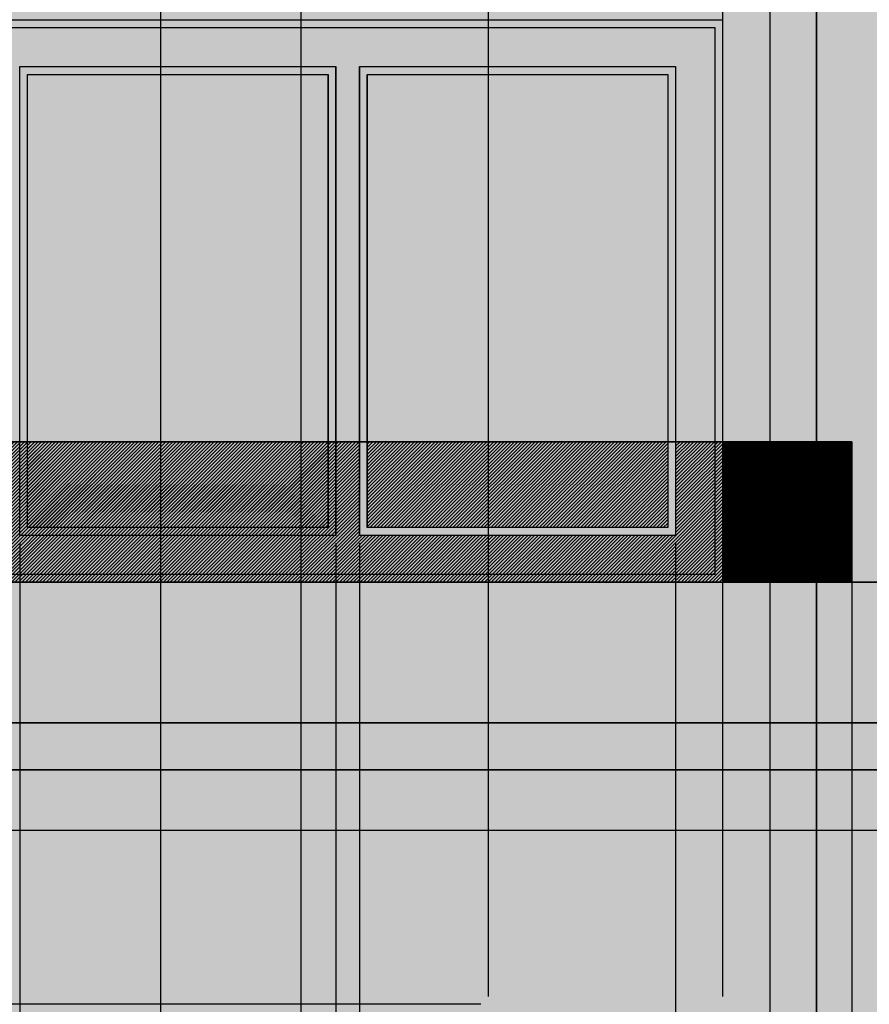
# Model space of a CAD drawing. Units: inches. Extents: x 860 to 1491, y 583 to 1370.
# Tile 5 of 8: x 998 to 1216, y 839 to 1091. Entities that reach past the tile are written whole.
import ezdxf

# ---------------------------------------------------------------- set-up
doc = ezdxf.new("R2010")
doc.units = ezdxf.units.IN
doc.header["$MEASUREMENT"] = 0
doc.layers.get('0').update_dxf_attribs({"color": 250})
for name, color, linetype, lineweight in [('A-ANNO-DIMS', 2, 'Continuous', 18), ('A-ELEV', 7, 'Continuous', 35), ('A-ELEV-PATT', 9, 'Continuous', 13), ('A-GLAZ', 4, 'Continuous', 25), ('A-GLAZ-PATT', 150, 'Continuous', 13), ('A-RAIL-PATT', 150, 'Continuous', 13)]:
    doc.layers.add(name, color=color, linetype=linetype, lineweight=lineweight)
doc.styles.get("Standard").update_dxf_attribs({"font": 'arial.ttf'})
doc.dimstyles.get("Standard").update_dxf_attribs({"dimtxt": 6, "dimasz": 0.18, "dimexe": 3, "dimexo": 2, "dimgap": 2, "dimtad": 0, "dimtih": 1, "dimtoh": 1, "dimdec": 0, "dimzin": 0, "dimdsep": 46, "dimlunit": 3, "dimtxsty": 'Standard', "dimblk2": 'CLOSEDBLANK', "dimsah": 1, "dimcen": 2, "dimadec": 0, "dimazin": 0, "dimtfac": 1, "dimtdec": 0, "dimtofl": 0, "dimtmove": 0, "dimatfit": 3, "dimfxl": 1, "dimtolj": 1, "dimtzin": 0, "dimarcsym": 0})

# ---------------------------------------------------------------- blocks, each defined once
blk = doc.blocks.new('_ClosedBlank')
at = {"color": 0, "linetype": 'ByBlock', "lineweight": -2}
for p, q in [((-1, 0.17), (0, 0)), ((-1, 0.17), (-1, -0.17)), ((0, 0), (-1, -0.17))]:
    blk.add_line(p, q, dxfattribs=at)
blk = doc.blocks.new('*D2')
at = {"layer": 'A-ANNO-DIMS', "color": 0, "lineweight": -2, "transparency": 16777216}
for p, q in [((1442.44, 1328.76), (1442.44, 584.11)), ((908.34, 740.76), (908.34, 584.11)), ((908.52, 587.11), (1163.85, 587.11)), ((1442.26, 587.11), (1186.93, 587.11))]:
    blk.add_line(p, q, dxfattribs=at)
at = {"layer": 'A-ANNO-DIMS', "color": 0, "transparency": 16777216}
blk.add_solid([(908.52, 587.14), (908.52, 587.08), (908.34, 587.11)], dxfattribs=at)
at = {"layer": 'Defpoints', "color": 0, "transparency": 16777216}
for p in [(1442.44, 1330.76), (908.34, 742.76), (1442.44, 587.11)]:
    blk.add_point(p, dxfattribs=at)
at = {"layer": 'A-ANNO-DIMS', "color": 0, "lineweight": -2, "transparency": 16777216, "xscale": 0.18, "yscale": 0.18, "zscale": 0.18}
blk.add_blockref('_ClosedBlank', (1442.44, 587.11), dxfattribs=at)
at = {"layer": 'A-ANNO-DIMS', "color": 0, "transparency": 16777216, "insert": (1175.39, 587.11), "char_height": 6, "attachment_point": 5}
blk.add_mtext('\\A1;534.1', dxfattribs=at)
blk = doc.blocks.new('*D21')
at = {"layer": 'A-ANNO-DIMS', "color": 0, "lineweight": -2, "transparency": 16777216}
for p, q in [((962.34, 732.76), (962.34, 1369.41)), ((1034.46, 828.76), (1034.46, 1369.41)), ((962.52, 1366.41), (986.33, 1366.41)), ((1034.28, 1366.41), (1010.47, 1366.41))]:
    blk.add_line(p, q, dxfattribs=at)
at = {"layer": 'A-ANNO-DIMS', "color": 0, "transparency": 16777216}
blk.add_solid([(962.52, 1366.44), (962.52, 1366.38), (962.34, 1366.41)], dxfattribs=at)
at = {"layer": 'Defpoints', "color": 0, "transparency": 16777216}
for p in [(1034.46, 1366.41), (1034.46, 826.76), (962.34, 730.76)]:
    blk.add_point(p, dxfattribs=at)
at = {"layer": 'A-ANNO-DIMS', "color": 0, "lineweight": -2, "transparency": 16777216, "xscale": 0.18, "yscale": 0.18, "zscale": 0.18}
blk.add_blockref('_ClosedBlank', (1034.46, 1366.41), dxfattribs=at)
at = {"layer": 'A-ANNO-DIMS', "color": 0, "transparency": 16777216, "insert": (998.4, 1366.41), "char_height": 6, "attachment_point": 5}
blk.add_mtext('\\A1;72.12', dxfattribs=at)
blk = doc.blocks.new('*D22')
at = {"layer": 'A-ANNO-DIMS', "color": 0, "lineweight": -2, "transparency": 16777216}
for p, q in [((1034.46, 828.76), (1034.46, 1369.41)), ((1070.46, 828.76), (1070.46, 1369.41)), ((1034.64, 1366.41), (1046.17, 1366.41)), ((1070.28, 1366.41), (1058.75, 1366.41))]:
    blk.add_line(p, q, dxfattribs=at)
at = {"layer": 'A-ANNO-DIMS', "color": 0, "transparency": 16777216}
blk.add_solid([(1034.64, 1366.44), (1034.64, 1366.38), (1034.46, 1366.41)], dxfattribs=at)
at = {"layer": 'Defpoints', "color": 0, "transparency": 16777216}
for p in [(1070.46, 1366.41), (1034.46, 826.76), (1070.46, 826.76)]:
    blk.add_point(p, dxfattribs=at)
at = {"layer": 'A-ANNO-DIMS', "color": 0, "lineweight": -2, "transparency": 16777216, "xscale": 0.18, "yscale": 0.18, "zscale": 0.18}
blk.add_blockref('_ClosedBlank', (1070.46, 1366.41), dxfattribs=at)
at = {"layer": 'A-ANNO-DIMS', "color": 0, "transparency": 16777216, "insert": (1052.46, 1366.41), "char_height": 6, "attachment_point": 5}
blk.add_mtext('\\A1;36', dxfattribs=at)
blk = doc.blocks.new('*D23')
at = {"layer": 'A-ANNO-DIMS', "color": 0, "lineweight": -2, "transparency": 16777216}
for p, q in [((1070.46, 828.76), (1070.46, 1369.41)), ((1118.44, 840.76), (1118.44, 1369.41)), ((1070.64, 1366.41), (1082.2, 1366.41)), ((1118.26, 1366.41), (1106.7, 1366.41))]:
    blk.add_line(p, q, dxfattribs=at)
at = {"layer": 'A-ANNO-DIMS', "color": 0, "transparency": 16777216}
blk.add_solid([(1070.64, 1366.44), (1070.64, 1366.38), (1070.46, 1366.41)], dxfattribs=at)
at = {"layer": 'Defpoints', "color": 0, "transparency": 16777216}
for p in [(1118.44, 1366.41), (1118.44, 838.76), (1070.46, 826.76)]:
    blk.add_point(p, dxfattribs=at)
at = {"layer": 'A-ANNO-DIMS', "color": 0, "lineweight": -2, "transparency": 16777216, "xscale": 0.18, "yscale": 0.18, "zscale": 0.18}
blk.add_blockref('_ClosedBlank', (1118.44, 1366.41), dxfattribs=at)
at = {"layer": 'A-ANNO-DIMS', "color": 0, "transparency": 16777216, "insert": (1094.45, 1366.41), "char_height": 6, "attachment_point": 5}
blk.add_mtext('\\A1;47.98', dxfattribs=at)
blk = doc.blocks.new('*D24')
at = {"layer": 'A-ANNO-DIMS', "color": 0, "lineweight": -2, "transparency": 16777216}
for p, q in [((1118.44, 840.76), (1118.44, 1369.41)), ((1178.44, 840.76), (1178.44, 1369.41)), ((1118.62, 1366.41), (1142.14, 1366.41)), ((1178.26, 1366.41), (1154.74, 1366.41))]:
    blk.add_line(p, q, dxfattribs=at)
at = {"layer": 'A-ANNO-DIMS', "color": 0, "transparency": 16777216}
blk.add_solid([(1118.62, 1366.44), (1118.62, 1366.38), (1118.44, 1366.41)], dxfattribs=at)
at = {"layer": 'Defpoints', "color": 0, "transparency": 16777216}
for p in [(1178.44, 1366.41), (1118.44, 838.76), (1178.44, 838.76)]:
    blk.add_point(p, dxfattribs=at)
at = {"layer": 'A-ANNO-DIMS', "color": 0, "lineweight": -2, "transparency": 16777216, "xscale": 0.18, "yscale": 0.18, "zscale": 0.18}
blk.add_blockref('_ClosedBlank', (1178.44, 1366.41), dxfattribs=at)
at = {"layer": 'A-ANNO-DIMS', "color": 0, "transparency": 16777216, "insert": (1148.44, 1366.41), "char_height": 6, "attachment_point": 5}
blk.add_mtext('\\A1;60', dxfattribs=at)
blk = doc.blocks.new('*D25')
at = {"layer": 'A-ANNO-DIMS', "color": 0, "lineweight": -2, "transparency": 16777216}
for p, q in [((1178.44, 840.76), (1178.44, 1369.41)), ((1202.44, 744.76), (1202.44, 1369.41)), ((1178.62, 1366.41), (1184.1, 1366.41)), ((1202.26, 1366.41), (1196.78, 1366.41))]:
    blk.add_line(p, q, dxfattribs=at)
at = {"layer": 'A-ANNO-DIMS', "color": 0, "transparency": 16777216}
blk.add_solid([(1178.62, 1366.44), (1178.62, 1366.38), (1178.44, 1366.41)], dxfattribs=at)
at = {"layer": 'Defpoints', "color": 0, "transparency": 16777216}
for p in [(1202.44, 1366.41), (1178.44, 838.76), (1202.44, 742.76)]:
    blk.add_point(p, dxfattribs=at)
at = {"layer": 'A-ANNO-DIMS', "color": 0, "lineweight": -2, "transparency": 16777216, "xscale": 0.18, "yscale": 0.18, "zscale": 0.18}
blk.add_blockref('_ClosedBlank', (1202.44, 1366.41), dxfattribs=at)
at = {"layer": 'A-ANNO-DIMS', "color": 0, "transparency": 16777216, "insert": (1190.44, 1366.41), "char_height": 6, "attachment_point": 5}
blk.add_mtext('\\A1;24', dxfattribs=at)
blk = doc.blocks.new('*D26')
at = {"layer": 'A-ANNO-DIMS', "color": 0, "lineweight": -2, "transparency": 16777216}
for p, q in [((1202.44, 744.76), (1202.44, 1369.41)), ((1268.44, 864.76), (1268.44, 1369.41)), ((1202.62, 1366.41), (1229.13, 1366.41)), ((1268.26, 1366.41), (1241.75, 1366.41))]:
    blk.add_line(p, q, dxfattribs=at)
at = {"layer": 'A-ANNO-DIMS', "color": 0, "transparency": 16777216}
blk.add_solid([(1202.62, 1366.44), (1202.62, 1366.38), (1202.44, 1366.41)], dxfattribs=at)
at = {"layer": 'Defpoints', "color": 0, "transparency": 16777216}
for p in [(1268.44, 1366.41), (1268.44, 862.76), (1202.44, 742.76)]:
    blk.add_point(p, dxfattribs=at)
at = {"layer": 'A-ANNO-DIMS', "color": 0, "lineweight": -2, "transparency": 16777216, "xscale": 0.18, "yscale": 0.18, "zscale": 0.18}
blk.add_blockref('_ClosedBlank', (1268.44, 1366.41), dxfattribs=at)
at = {"layer": 'A-ANNO-DIMS', "color": 0, "transparency": 16777216, "insert": (1235.44, 1366.41), "char_height": 6, "attachment_point": 5}
blk.add_mtext('\\A1;66', dxfattribs=at)
blk = doc.blocks.new('*D35')
at = {"layer": 'A-ANNO-DIMS', "color": 0, "lineweight": -2, "transparency": 16777216}
for p, q in [((1116.440309, 838.755507), (869.690309, 838.755507)), ((872.690309, 838.935507), (872.690309, 839.115507)), ((1032.458453, 826.755507), (869.690309, 826.755507)), ((872.690309, 826.575507), (872.690309, 826.395507))]:
    blk.add_line(p, q, dxfattribs=at)
at = {"layer": 'A-ANNO-DIMS', "color": 0, "transparency": 16777216}
blk.add_solid([(872.660309, 826.575507), (872.720309, 826.575507), (872.690309, 826.755507)], dxfattribs=at)
at = {"layer": 'Defpoints', "color": 0, "transparency": 16777216}
for p in [(872.690309, 838.755507), (1118.440309, 838.755507), (1034.458453, 826.755507)]:
    blk.add_point(p, dxfattribs=at)
at = {"layer": 'A-ANNO-DIMS', "color": 0, "lineweight": -2, "transparency": 16777216, "xscale": 0.18, "yscale": 0.18, "zscale": 0.18, "rotation": 270}
blk.add_blockref('_ClosedBlank', (872.690309, 838.755507), dxfattribs=at)
at = {"layer": 'A-ANNO-DIMS', "color": 0, "transparency": 16777216, "insert": (872.690309, 832.755507), "char_height": 6, "attachment_point": 5}
blk.add_mtext('\\A1;12', dxfattribs=at)
blk = doc.blocks.new('*D48')
at = {"layer": 'A-ANNO-DIMS', "color": 0, "lineweight": -2, "transparency": 16777216}
for p, q in [((1222.44, 898.76), (1481.09, 898.76)), ((1478.09, 898.58), (1478.09, 896.12)), ((1478.09, 883.53), (1478.09, 885.99)), ((964.34, 883.35), (1481.09, 883.35))]:
    blk.add_line(p, q, dxfattribs=at)
at = {"layer": 'A-ANNO-DIMS', "color": 0, "transparency": 16777216}
blk.add_solid([(1478.06, 883.53), (1478.12, 883.53), (1478.09, 883.35)], dxfattribs=at)
at = {"layer": 'Defpoints', "color": 0, "transparency": 16777216}
for p in [(1220.44, 898.76), (1478.09, 898.76), (962.34, 883.35)]:
    blk.add_point(p, dxfattribs=at)
at = {"layer": 'A-ANNO-DIMS', "color": 0, "lineweight": -2, "transparency": 16777216, "xscale": 0.18, "yscale": 0.18, "zscale": 0.18, "rotation": 90}
blk.add_blockref('_ClosedBlank', (1478.09, 898.76), dxfattribs=at)
at = {"layer": 'A-ANNO-DIMS', "color": 0, "transparency": 16777216, "insert": (1478.09, 891.05), "char_height": 6, "attachment_point": 5}
blk.add_mtext('\\A1;15.402', dxfattribs=at)
blk = doc.blocks.new('*D65')
at = {"layer": 'A-ANNO-DIMS', "color": 0, "lineweight": -2, "transparency": 16777216}
for p, q in [((998.34, 956.76), (998.34, 584.11)), ((1079.34, 956.76), (1079.34, 584.11)), ((998.52, 587.11), (1033.12, 587.11)), ((1079.16, 587.11), (1044.56, 587.11))]:
    blk.add_line(p, q, dxfattribs=at)
at = {"layer": 'A-ANNO-DIMS', "color": 0, "transparency": 16777216}
blk.add_solid([(998.52, 587.14), (998.52, 587.08), (998.34, 587.11)], dxfattribs=at)
at = {"layer": 'Defpoints', "color": 0, "transparency": 16777216}
for p in [(998.34, 958.76), (1079.34, 958.76), (1079.34, 587.11)]:
    blk.add_point(p, dxfattribs=at)
at = {"layer": 'A-ANNO-DIMS', "color": 0, "lineweight": -2, "transparency": 16777216, "xscale": 0.18, "yscale": 0.18, "zscale": 0.18}
blk.add_blockref('_ClosedBlank', (1079.34, 587.11), dxfattribs=at)
at = {"layer": 'A-ANNO-DIMS', "color": 0, "transparency": 16777216, "insert": (1038.84, 587.11), "char_height": 6, "attachment_point": 5}
blk.add_mtext('\\A1;81', dxfattribs=at)
blk = doc.blocks.new('*D66')
at = {"layer": 'A-ANNO-DIMS', "color": 0, "lineweight": -2, "transparency": 16777216}
for p, q in [((1079.34, 956.76), (1079.34, 584.11)), ((1085.34, 956.76), (1085.34, 584.11)), ((1079.52, 587.11), (1085.16, 587.11)), ((1085.34, 587.11), (1085.52, 587.11))]:
    blk.add_line(p, q, dxfattribs=at)
at = {"layer": 'A-ANNO-DIMS', "color": 0, "transparency": 16777216}
blk.add_solid([(1079.52, 587.14), (1079.52, 587.08), (1079.34, 587.11)], dxfattribs=at)
at = {"layer": 'Defpoints', "color": 0, "transparency": 16777216}
for p in [(1079.34, 958.76), (1085.34, 958.76), (1085.34, 587.11)]:
    blk.add_point(p, dxfattribs=at)
at = {"layer": 'A-ANNO-DIMS', "color": 0, "lineweight": -2, "transparency": 16777216, "xscale": 0.18, "yscale": 0.18, "zscale": 0.18}
blk.add_blockref('_ClosedBlank', (1085.34, 587.11), dxfattribs=at)
at = {"layer": 'A-ANNO-DIMS', "color": 0, "transparency": 16777216, "insert": (1089.5, 587.11), "char_height": 6, "attachment_point": 5}
blk.add_mtext('\\A1;6', dxfattribs=at)
blk = doc.blocks.new('*D67')
at = {"layer": 'A-ANNO-DIMS', "color": 0, "lineweight": -2, "transparency": 16777216}
for p, q in [((1085.34, 956.76), (1085.34, 584.11)), ((1166.34, 956.76), (1166.34, 584.11)), ((1085.52, 587.11), (1120.12, 587.11)), ((1166.16, 587.11), (1131.56, 587.11))]:
    blk.add_line(p, q, dxfattribs=at)
at = {"layer": 'A-ANNO-DIMS', "color": 0, "transparency": 16777216}
blk.add_solid([(1085.52, 587.14), (1085.52, 587.08), (1085.34, 587.11)], dxfattribs=at)
at = {"layer": 'Defpoints', "color": 0, "transparency": 16777216}
for p in [(1085.34, 958.76), (1166.34, 958.76), (1166.34, 587.11)]:
    blk.add_point(p, dxfattribs=at)
at = {"layer": 'A-ANNO-DIMS', "color": 0, "lineweight": -2, "transparency": 16777216, "xscale": 0.18, "yscale": 0.18, "zscale": 0.18}
blk.add_blockref('_ClosedBlank', (1166.34, 587.11), dxfattribs=at)
at = {"layer": 'A-ANNO-DIMS', "color": 0, "transparency": 16777216, "insert": (1125.84, 587.11), "char_height": 6, "attachment_point": 5}
blk.add_mtext('\\A1;81', dxfattribs=at)
blk = doc.blocks.new('*D68')
at = {"layer": 'A-ANNO-DIMS', "color": 0, "lineweight": -2, "transparency": 16777216}
for p, q in [((1211.44, 980.76), (1211.44, 584.11)), ((1166.34, 956.76), (1166.34, 584.11)), ((1166.52, 587.11), (1179.56, 587.11)), ((1211.26, 587.11), (1198.22, 587.11))]:
    blk.add_line(p, q, dxfattribs=at)
at = {"layer": 'A-ANNO-DIMS', "color": 0, "transparency": 16777216}
blk.add_solid([(1166.52, 587.14), (1166.52, 587.08), (1166.34, 587.11)], dxfattribs=at)
at = {"layer": 'Defpoints', "color": 0, "transparency": 16777216}
for p in [(1211.44, 982.76), (1166.34, 958.76), (1211.44, 587.11)]:
    blk.add_point(p, dxfattribs=at)
at = {"layer": 'A-ANNO-DIMS', "color": 0, "lineweight": -2, "transparency": 16777216, "xscale": 0.18, "yscale": 0.18, "zscale": 0.18}
blk.add_blockref('_ClosedBlank', (1211.44, 587.11), dxfattribs=at)
at = {"layer": 'A-ANNO-DIMS', "color": 0, "transparency": 16777216, "insert": (1188.89, 587.11), "char_height": 6, "attachment_point": 5}
blk.add_mtext('\\A1;45.1', dxfattribs=at)
blk = doc.blocks.new('*D69')
at = {"layer": 'A-ANNO-DIMS', "color": 0, "lineweight": -2, "transparency": 16777216}
for p, q in [((1211.440309, 980.755507), (1211.440309, 584.105507)), ((1220.440309, 896.755507), (1220.440309, 584.105507)), ((1211.260309, 587.105507), (1211.080309, 587.105507)), ((1220.620309, 587.105507), (1220.800309, 587.105507))]:
    blk.add_line(p, q, dxfattribs=at)
at = {"layer": 'A-ANNO-DIMS', "color": 0, "transparency": 16777216}
blk.add_solid([(1211.260309, 587.135507), (1211.260309, 587.075507), (1211.440309, 587.105507)], dxfattribs=at)
at = {"layer": 'Defpoints', "color": 0, "transparency": 16777216}
for p in [(1211.440309, 982.755507), (1220.440309, 898.755507), (1220.440309, 587.105507)]:
    blk.add_point(p, dxfattribs=at)
at = {"layer": 'A-ANNO-DIMS', "color": 0, "lineweight": -2, "transparency": 16777216, "xscale": 0.18, "yscale": 0.18, "zscale": 0.18, "rotation": 180}
blk.add_blockref('_ClosedBlank', (1220.440309, 587.105507), dxfattribs=at)
at = {"layer": 'A-ANNO-DIMS', "color": 0, "transparency": 16777216, "insert": (1215.940309, 587.105507), "char_height": 6, "attachment_point": 5}
blk.add_mtext('\\A1;9', dxfattribs=at)
blk = doc.blocks.new('*D76')
at = {"layer": 'A-ANNO-DIMS', "color": 0, "lineweight": -2, "transparency": 16777216}
for p, q in [((1202.440309, 1277.755507), (1202.440309, 584.105507)), ((1190.440309, 1214.755507), (1190.440309, 584.105507)), ((1190.260309, 587.105507), (1190.080309, 587.105507)), ((1202.620309, 587.105507), (1202.800309, 587.105507))]:
    blk.add_line(p, q, dxfattribs=at)
at = {"layer": 'A-ANNO-DIMS', "color": 0, "transparency": 16777216}
blk.add_solid([(1190.260309, 587.135507), (1190.260309, 587.075507), (1190.440309, 587.105507)], dxfattribs=at)
at = {"layer": 'Defpoints', "color": 0, "transparency": 16777216}
for p in [(1202.440309, 1279.755507), (1190.440309, 1216.755507), (1202.440309, 587.105507)]:
    blk.add_point(p, dxfattribs=at)
at = {"layer": 'A-ANNO-DIMS', "color": 0, "lineweight": -2, "transparency": 16777216, "xscale": 0.18, "yscale": 0.18, "zscale": 0.18, "rotation": 180}
blk.add_blockref('_ClosedBlank', (1202.440309, 587.105507), dxfattribs=at)
at = {"layer": 'A-ANNO-DIMS', "color": 0, "transparency": 16777216, "insert": (1196.440309, 587.105507), "char_height": 6, "attachment_point": 5}
blk.add_mtext('\\A1;12', dxfattribs=at)
blk = doc.blocks.new('*D77')
at = {"layer": 'A-ANNO-DIMS', "color": 0, "lineweight": -2, "transparency": 16777216}
for p, q in [((1202.44, 1277.76), (1202.44, 584.11)), ((1352.44, 1277.76), (1352.44, 584.11)), ((1202.62, 587.11), (1269.1, 587.11)), ((1352.26, 587.11), (1285.78, 587.11))]:
    blk.add_line(p, q, dxfattribs=at)
at = {"layer": 'A-ANNO-DIMS', "color": 0, "transparency": 16777216}
blk.add_solid([(1202.62, 587.14), (1202.62, 587.08), (1202.44, 587.11)], dxfattribs=at)
at = {"layer": 'Defpoints', "color": 0, "transparency": 16777216}
for p in [(1202.44, 1279.76), (1352.44, 1279.76), (1352.44, 587.11)]:
    blk.add_point(p, dxfattribs=at)
at = {"layer": 'A-ANNO-DIMS', "color": 0, "lineweight": -2, "transparency": 16777216, "xscale": 0.18, "yscale": 0.18, "zscale": 0.18}
blk.add_blockref('_ClosedBlank', (1352.44, 587.11), dxfattribs=at)
at = {"layer": 'A-ANNO-DIMS', "color": 0, "transparency": 16777216, "insert": (1277.44, 587.11), "char_height": 6, "attachment_point": 5}
blk.add_mtext('\\A1;150', dxfattribs=at)

msp = doc.modelspace()

# ---------------------------------------------------------------- hatches: boundary and pattern name
at = {"layer": 'A-ELEV-PATT'}
h = msp.add_hatch(color=256, dxfattribs=at)
h.dxf.hatch_style = 1
h.paths.add_polyline_path([(1442.4403, 1330.7555), (1370.4403, 1330.7555), (1370.4403, 622.7555), (1442.4403, 622.7555)])
h.paths.add_polyline_path([(1358.4403, 1306.7555), (1190.4403, 1306.7555), (1190.4403, 1288.7555), (1358.4403, 1288.7555)])
h.paths.add_polyline_path([(1190.4403, 1234.7555), (962.3403, 1234.7555), (962.3403, 1198.7555), (1202.4403, 1198.7555), (1202.4403, 1216.7555), (1190.4403, 1216.7555)])
h.paths.add_polyline_path([(1202.4403, 1117.6207), (962.3403, 1117.6207), (962.3403, 982.7555), (986.3403, 982.7555), (986.3403, 1090.7555), (1178.3403, 1090.7555), (1178.3403, 982.7555), (1202.4403, 982.7555)])
h.paths.add_polyline_path([(1319.4403, 1184.7555), (1202.4403, 1184.7555), (1202.4403, 982.7555), (1211.4403, 982.7555), (1211.4403, 946.7555), (1220.4403, 946.7555), (1220.4403, 934.7555), (1319.4403, 934.7555)])
h.paths.add_polyline_path([(1271.4403, 1160.7555), (1307.4403, 1160.7555), (1307.4403, 944.7555), (1271.4403, 944.7555)], flags=16)
h.paths.add_polyline_path([(1275.4403, 1156.7555), (1303.4403, 1156.7555), (1303.4403, 948.7555), (1275.4403, 948.7555)], flags=0)
h.paths.add_polyline_path([(1202.4403, 898.7555), (962.3403, 898.7555), (962.3403, 730.7555), (1034.4585, 730.7555), (1034.4585, 826.7555), (1070.4585, 826.7555), (1070.4585, 730.7555), (1118.4403, 730.7555), (1118.4403, 838.7555), (1178.4403, 838.7555), (1178.4403, 730.7555), (1202.4403, 730.7555)])
h.paths.add_polyline_path([(1220.4403, 946.7555), (1211.4403, 946.7555), (938.3403, 946.7555), (926.3403, 946.7555), (926.3403, 910.7555), (962.3403, 910.7555), (1220.4403, 910.7555)])
h.paths.add_polyline_path([(950.3403, 730.7555), (950.3403, 734.7555), (938.3403, 742.7555), (938.3403, 730.7555), (938.3403, 622.7555), (950.3403, 622.7555)])
h = msp.add_hatch(color=256, dxfattribs=at)
h.dxf.hatch_style = 1
h.paths.add_polyline_path([(1352.4403, 1279.7555), (1202.4403, 1279.7555), (1202.4403, 1198.7555), (1328.4403, 1198.7555), (1328.4403, 922.7555), (1220.4403, 922.7555), (1220.4403, 898.7555), (1202.4403, 898.7555), (1202.4403, 742.7555), (1232.4403, 742.7555), (1232.4403, 730.7555), (1352.4403, 730.7555)])
h.paths.add_polyline_path([(1268.4403, 862.7555), (1340.4403, 862.7555), (1340.4403, 790.7555), (1268.4403, 790.7555)], flags=16)
h.paths.add_polyline_path([(1272.4403, 858.7555), (1302.4403, 858.7555), (1302.4403, 794.7555), (1272.4403, 794.7555)], flags=0)
h.paths.add_polyline_path([(1306.4403, 858.7555), (1336.4403, 858.7555), (1336.4403, 794.7555), (1306.4403, 794.7555)], flags=0)
h = msp.add_hatch(color=256, dxfattribs=at)
h.paths.add_polyline_path([(1176.3403, 1088.7555), (988.3403, 1088.7555), (988.3403, 982.7555), (998.3403, 982.7555), (998.3403, 1078.7555), (1079.3403, 1078.7555), (1079.3403, 982.7555), (1085.3403, 982.7555), (1085.3403, 1078.7555), (1166.3403, 1078.7555), (1166.3403, 982.7555), (1176.3403, 982.7555)])
h.paths.add_polyline_path([(1176.3403, 982.7555), (1166.3403, 982.7555), (1166.3403, 958.7555), (1085.3403, 958.7555), (1085.3403, 982.7555), (1079.3403, 982.7555), (1079.3403, 958.7555), (998.3403, 958.7555), (998.3403, 982.7555), (988.3403, 982.7555), (988.3403, 948.7555), (1176.3403, 948.7555)])
h.paths.add_polyline_path([(1307.4403, 1160.7555), (1271.4403, 1160.7555), (1271.4403, 944.7555), (1307.4403, 944.7555)])
h.paths.add_polyline_path([(1275.4403, 1156.7555), (1303.4403, 1156.7555), (1303.4403, 948.7555), (1275.4403, 948.7555)], flags=16)
h.paths.add_polyline_path([(1340.4403, 862.7555), (1268.4403, 862.7555), (1268.4403, 790.7555), (1340.4403, 790.7555)])
h.paths.add_polyline_path([(1306.4403, 794.7555), (1306.4403, 858.7555), (1336.4403, 858.7555), (1336.4403, 794.7555)], flags=16)
h.paths.add_polyline_path([(1302.4403, 794.7555), (1272.4403, 794.7555), (1272.4403, 858.7555), (1302.4403, 858.7555)], flags=16)
h.paths.add_polyline_path([(1124.4403, 832.7555), (1172.4403, 832.7555), (1172.4403, 730.7555), (1178.4403, 730.7555), (1178.4403, 838.7555), (1118.4403, 838.7555), (1118.4403, 742.7555), (1124.4403, 742.7555), (1124.4403, 766.7555)])
h.paths.add_polyline_path([(1070.4585, 826.7555), (1034.4585, 826.7555), (1034.4585, 730.7555), (1070.4585, 730.7555)])
h.paths.add_polyline_path([(1066.4585, 822.7555), (1066.4585, 734.7555), (1038.4585, 734.7555), (1038.4585, 822.7555)], flags=16)
h.paths.add_polyline_path([(1129.9403, 766.7555, 1), (1124.9403, 766.7555, 1)], flags=17)
h = msp.add_hatch(color=256, dxfattribs=at)
h.dxf.hatch_style = 1
h.paths.add_polyline_path([(1220.4403, 910.7555), (938.3403, 910.7555), (926.3403, 910.7555), (962.3403, 883.3536), (962.3403, 898.7555), (1220.4403, 898.7555)])
at = {"layer": 'A-GLAZ-PATT'}
h = msp.add_hatch(color=256, dxfattribs=at)
h.paths.add_polyline_path([(1178.3403, 982.7555), (1176.3403, 982.7555), (1176.3403, 948.7555), (988.3403, 948.7555), (988.3403, 982.7555), (986.3403, 982.7555), (986.3403, 946.7555), (1178.3403, 946.7555)])
h.paths.add_polyline_path([(1178.3403, 1090.7555), (986.3403, 1090.7555), (986.3403, 982.7555), (988.3403, 982.7555), (988.3403, 1088.7555), (1176.3403, 1088.7555), (1176.3403, 982.7555), (1178.3403, 982.7555)])
h.paths.add_polyline_path([(1124.4403, 766.7555, 1), (1130.4403, 766.7555, 1)])
h.paths.add_polyline_path([(1129.9403, 766.7555, -1), (1124.9403, 766.7555, -1)], flags=16)
h = msp.add_hatch(color=256, dxfattribs=at)
h.paths.add_polyline_path([(1166.3403, 1078.7555), (1085.3403, 1078.7555), (1085.3403, 958.7555), (1166.3403, 958.7555)])
h.paths.add_polyline_path([(1087.3403, 1076.7555), (1164.3403, 1076.7555), (1164.3403, 960.7555), (1087.3403, 960.7555)], flags=16)
h.paths.add_polyline_path([(1079.3403, 1078.7555), (998.3403, 1078.7555), (998.3403, 958.7555), (1079.3403, 958.7555)])
h.paths.add_polyline_path([(1077.3403, 1076.7555), (1077.3403, 960.7555), (1000.3403, 960.7555), (1000.3403, 1076.7555)], flags=16)
h = msp.add_hatch(color=256, dxfattribs=at)
h.set_gradient(color1=(51, 167, 230), color2=(122, 175, 223), name='CYLINDER')
h.paths.add_polyline_path([(1000.3403, 982.7555), (1077.3403, 982.7555), (1077.3403, 1076.7555), (1000.3403, 1076.7555)])
h = msp.add_hatch(color=256, dxfattribs=at)
h.set_gradient(color1=(51, 167, 230), color2=(122, 175, 223), name='CYLINDER')
h.paths.add_polyline_path([(1164.3403, 1076.7555), (1087.3403, 1076.7555), (1087.3403, 982.7555), (1164.3403, 982.7555)])
h.paths.add_polyline_path([(1164.3403, 982.7555), (1087.3403, 982.7555), (1087.3403, 960.7555), (1164.3403, 960.7555)])
h = msp.add_hatch(color=256, dxfattribs=at)
h.set_gradient(color1=(51, 167, 230), color2=(122, 175, 223), name='CYLINDER')
h.paths.add_polyline_path([(1077.3403, 960.7555), (1077.3403, 982.7555), (1000.3403, 982.7555), (1000.3403, 960.7555)])
at = {"layer": 'A-RAIL-PATT'}
h = msp.add_hatch(dxfattribs=at)
h.set_pattern_fill('ANSI31', color=256, style=0)
h.paths.add_polyline_path([(1211.4403, 982.7555), (1202.4403, 982.7555), (1202.4403, 946.7555), (1211.4403, 946.7555)])
h.paths.add_polyline_path([(1202.4403, 982.7555), (1178.3403, 982.7555), (1178.3403, 946.7555), (1202.4403, 946.7555)])
h.paths.add_polyline_path([(986.3403, 982.7555), (962.3403, 982.7555), (962.3403, 946.7555), (986.3403, 946.7555)])
h.paths.add_polyline_path([(962.3403, 982.7555), (938.3403, 982.7555), (962.3403, 946.7555)], flags=17)
h.paths.add_polyline_path([(938.3403, 982.7555), (938.3403, 946.7555), (962.3403, 946.7555)])
h = msp.add_hatch(dxfattribs=at)
h.set_pattern_fill('ANSI31', color=256, scale=5, style=0)
h.paths.add_polyline_path([(962.3403, 982.7555), (938.3403, 982.7555), (962.3403, 946.7555)], flags=17)
h.paths.add_polyline_path([(938.3403, 982.7555), (938.3403, 946.7555), (962.3403, 946.7555)])
h.paths.add_polyline_path([(986.3403, 982.7555), (962.3403, 982.7555), (962.3403, 946.7555), (986.3403, 946.7555)])
h.paths.add_polyline_path([(998.3403, 982.7555), (988.3403, 982.7555), (988.3403, 948.7555), (1176.3403, 948.7555), (1176.3403, 982.7555), (1166.3403, 982.7555), (1166.3403, 958.7555), (1085.3403, 958.7555), (1085.3403, 982.7555), (1079.3403, 982.7555), (1079.3403, 958.7555), (998.3403, 958.7555)], flags=17)
h.paths.add_polyline_path([(1000.3403, 982.7555), (998.3403, 982.7555), (998.3403, 958.7555), (1079.3403, 958.7555), (1079.3403, 982.7555), (1077.3403, 982.7555), (1077.3403, 960.7555), (1000.3403, 960.7555)], flags=16)
h.paths.add_polyline_path([(988.3403, 982.7555), (986.3403, 982.7555), (986.3403, 946.7555), (1178.3403, 946.7555), (1178.3403, 982.7555), (1176.3403, 982.7555), (1176.3403, 948.7555), (988.3403, 948.7555)])
h.paths.add_polyline_path([(1077.3403, 982.7555), (1000.3403, 982.7555), (1000.3403, 960.7555), (1077.3403, 960.7555)], flags=0)
h.paths.add_polyline_path([(1164.3403, 982.7555), (1087.3403, 982.7555), (1087.3403, 960.7555), (1164.3403, 960.7555)], flags=16)
h.paths.add_polyline_path([(1202.4403, 982.7555), (1178.3403, 982.7555), (1178.3403, 946.7555), (1202.4403, 946.7555)])
h = msp.add_hatch(dxfattribs=at)
h.set_pattern_fill('ANSI31', color=256, scale=5, style=0)
h.paths.add_polyline_path([(1077.3403, 982.7555), (1000.3403, 982.7555), (1000.3403, 960.7555), (1077.3403, 960.7555)])
h = msp.add_hatch(dxfattribs=at)
h.set_pattern_fill('ANSI31', color=256, scale=5, style=0)
h.paths.add_polyline_path([(1164.3403, 982.7555), (1087.3403, 982.7555), (1087.3403, 960.7555), (1164.3403, 960.7555)])
h = msp.add_hatch(dxfattribs=at)
h.set_pattern_fill('ANSI31', color=256, scale=5, style=0)
h.paths.add_polyline_path([(1211.4403, 982.7555), (1202.4403, 982.7555), (1202.4403, 946.7555), (1211.4403, 946.7555)])

# ---------------------------------------------------------------- linework, layer by layer
at = {"layer": 'A-ELEV'}
for p, q in [((1202.4403, 946.7555), (1202.4403, 1184.7555)), ((1079.3403, 1078.7555), (1079.3403, 958.7555)), ((1085.3403, 1078.7555), (1085.3403, 958.7555)), ((1077.3403, 1076.7555), (1077.3403, 960.7555)), ((1087.3403, 1076.7555), (1087.3403, 960.7555)), ((938.3403, 982.7555), (1211.4403, 982.7555)), ((1211.4403, 982.7555), (1211.4403, 946.7555)), ((938.3403, 946.7555), (1220.4403, 946.7555)), ((938.3403, 910.7555), (1220.4403, 910.7555)), ((962.3403, 898.7555), (1220.4403, 898.7555)), ((1202.4403, 622.7555), (1202.4403, 898.7555))]:
    msp.add_line(p, q, dxfattribs=at)
at = {"layer": 'A-GLAZ'}
for points in [[(986.3403, 1090.7555), (1178.3403, 1090.7555), (1178.3403, 946.7555), (986.3403, 946.7555)], [(988.3403, 1088.7555), (1176.3403, 1088.7555), (1176.3403, 948.7555), (988.3403, 948.7555)]]:
    msp.add_lwpolyline(points, close=True, dxfattribs=at)
for points in [[(1079.3403, 958.7555), (998.3403, 958.7555), (998.3403, 1078.7555), (1079.3403, 1078.7555)], [(1085.3403, 1078.7555), (1166.3403, 1078.7555), (1166.3403, 958.7555), (1085.3403, 958.7555)], [(1077.3403, 960.7555), (1000.3403, 960.7555), (1000.3403, 1076.7555), (1077.3403, 1076.7555)], [(1087.3403, 1076.7555), (1164.3403, 1076.7555), (1164.3403, 960.7555), (1087.3403, 960.7555)]]:
    msp.add_lwpolyline(points, dxfattribs=at)

# ---------------------------------------------------------------- dimensions: what is measured, and where the dimension line sits
at = {"layer": 'A-ANNO-DIMS'}
for base, p1, p2, override, picture, middle in [((1034.4585, 1366.4055), (962.3403, 730.7555), (1034.4585, 826.7555), {"dimdec": 2, "dimlfac": 1, "dimrnd": 0, "dimzin": 0, "dimdsep": 46, "dimlunit": 2}, '*D21', (998.3994, 1366.4055)), ((1070.4585, 1366.4055), (1034.4585, 826.7555), (1070.4585, 826.7555), {"dimdec": 0, "dimlfac": 1, "dimrnd": 0, "dimzin": 0, "dimdsep": 46, "dimlunit": 2}, '*D22', (1052.4585, 1366.4055)), ((1118.4403, 1366.4055), (1070.4585, 826.7555), (1118.4403, 838.7555), {"dimdec": 2, "dimlfac": 1, "dimrnd": 0, "dimzin": 0, "dimdsep": 46, "dimlunit": 2}, '*D23', (1094.4494, 1366.4055)), ((1178.4403, 1366.4055), (1118.4403, 838.7555), (1178.4403, 838.7555), {"dimdec": 0, "dimlfac": 1, "dimrnd": 0, "dimzin": 0, "dimdsep": 46, "dimlunit": 2}, '*D24', (1148.4403, 1366.4055)), ((1202.4403, 1366.4055), (1178.4403, 838.7555), (1202.4403, 742.7555), {"dimdec": 0, "dimlfac": 1, "dimrnd": 0, "dimzin": 0, "dimdsep": 46, "dimlunit": 2}, '*D25', (1190.4403, 1366.4055)), ((1268.4403, 1366.4055), (1202.4403, 742.7555), (1268.4403, 862.7555), {"dimdec": 0, "dimlfac": 1, "dimrnd": 0, "dimzin": 0, "dimdsep": 46, "dimlunit": 2}, '*D26', (1235.4403, 1366.4055)), ((1442.4403, 587.1055), (908.3403, 742.7555), (1442.4403, 1330.7555), {"dimdec": 1, "dimlfac": 1, "dimrnd": 0, "dimzin": 0, "dimdsep": 46, "dimlunit": 2}, '*D2', (1175.3903, 587.1055)), ((1202.4403, 587.1055), (1190.4403, 1216.7555), (1202.4403, 1279.7555), {"dimdec": 0, "dimlfac": 1, "dimrnd": 0, "dimzin": 0, "dimdsep": 46, "dimlunit": 2}, '*D76', (1196.4403, 587.1055)), ((1352.4403, 587.1055), (1202.4403, 1279.7555), (1352.4403, 1279.7555), {"dimdec": 0, "dimlfac": 1, "dimrnd": 0, "dimzin": 0, "dimdsep": 46, "dimlunit": 2}, '*D77', (1277.4403, 587.1055)), ((1211.4403, 587.1055), (1166.3403, 958.7555), (1211.4403, 982.7555), {"dimdec": 1, "dimlfac": 1, "dimrnd": 0, "dimzin": 0, "dimdsep": 46, "dimlunit": 2}, '*D68', (1188.8903, 587.1055)), ((1220.4403, 587.1055), (1211.4403, 982.7555), (1220.4403, 898.7555), {"dimdec": 0, "dimlfac": 1, "dimrnd": 0, "dimzin": 0, "dimdsep": 46, "dimlunit": 2}, '*D69', (1215.9403, 587.1055)), ((1079.3403, 587.1055), (998.3403, 958.7555), (1079.3403, 958.7555), {"dimdec": 0, "dimlfac": 1, "dimrnd": 0, "dimzin": 0, "dimdsep": 46, "dimlunit": 2}, '*D65', (1038.8403, 587.1055)), ((1085.3403, 587.1055), (1079.3403, 958.7555), (1085.3403, 958.7555), {"dimdec": 0, "dimlfac": 1, "dimrnd": 0, "dimzin": 0, "dimdsep": 46, "dimlunit": 2}, '*D66', (1089.5012, 587.1055)), ((1166.3403, 587.1055), (1085.3403, 958.7555), (1166.3403, 958.7555), {"dimdec": 0, "dimlfac": 1, "dimrnd": 0, "dimzin": 0, "dimdsep": 46, "dimlunit": 2}, '*D67', (1125.8403, 587.1055))]:
    dim = msp.add_linear_dim(base=base, p1=p1, p2=p2, dimstyle='Standard', override=override, dxfattribs=at)
    dim.commit()
    dim.dimension.update_dxf_attribs({"geometry": picture, "text_midpoint": middle})
for base, p1, p2, override, picture, middle in [((1478.0903, 898.7555), (962.3403, 883.3536), (1220.4403, 898.7555), {"dimdec": 3, "dimlfac": 1, "dimrnd": 0, "dimzin": 0, "dimdsep": 46, "dimlunit": 2}, '*D48', (1478.0903, 891.0545)), ((872.6903, 838.7555), (1034.4585, 826.7555), (1118.4403, 838.7555), {"dimdec": 0, "dimlfac": 1, "dimrnd": 0, "dimzin": 0, "dimdsep": 46, "dimlunit": 2}, '*D35', (872.6903, 832.7555))]:
    dim = msp.add_linear_dim(base=base, p1=p1, p2=p2, angle=90, dimstyle='Standard', override=override, dxfattribs=at)
    dim.commit()
    dim.dimension.update_dxf_attribs({"geometry": picture, "text_midpoint": middle})

doc.saveas('drawing.dxf')
